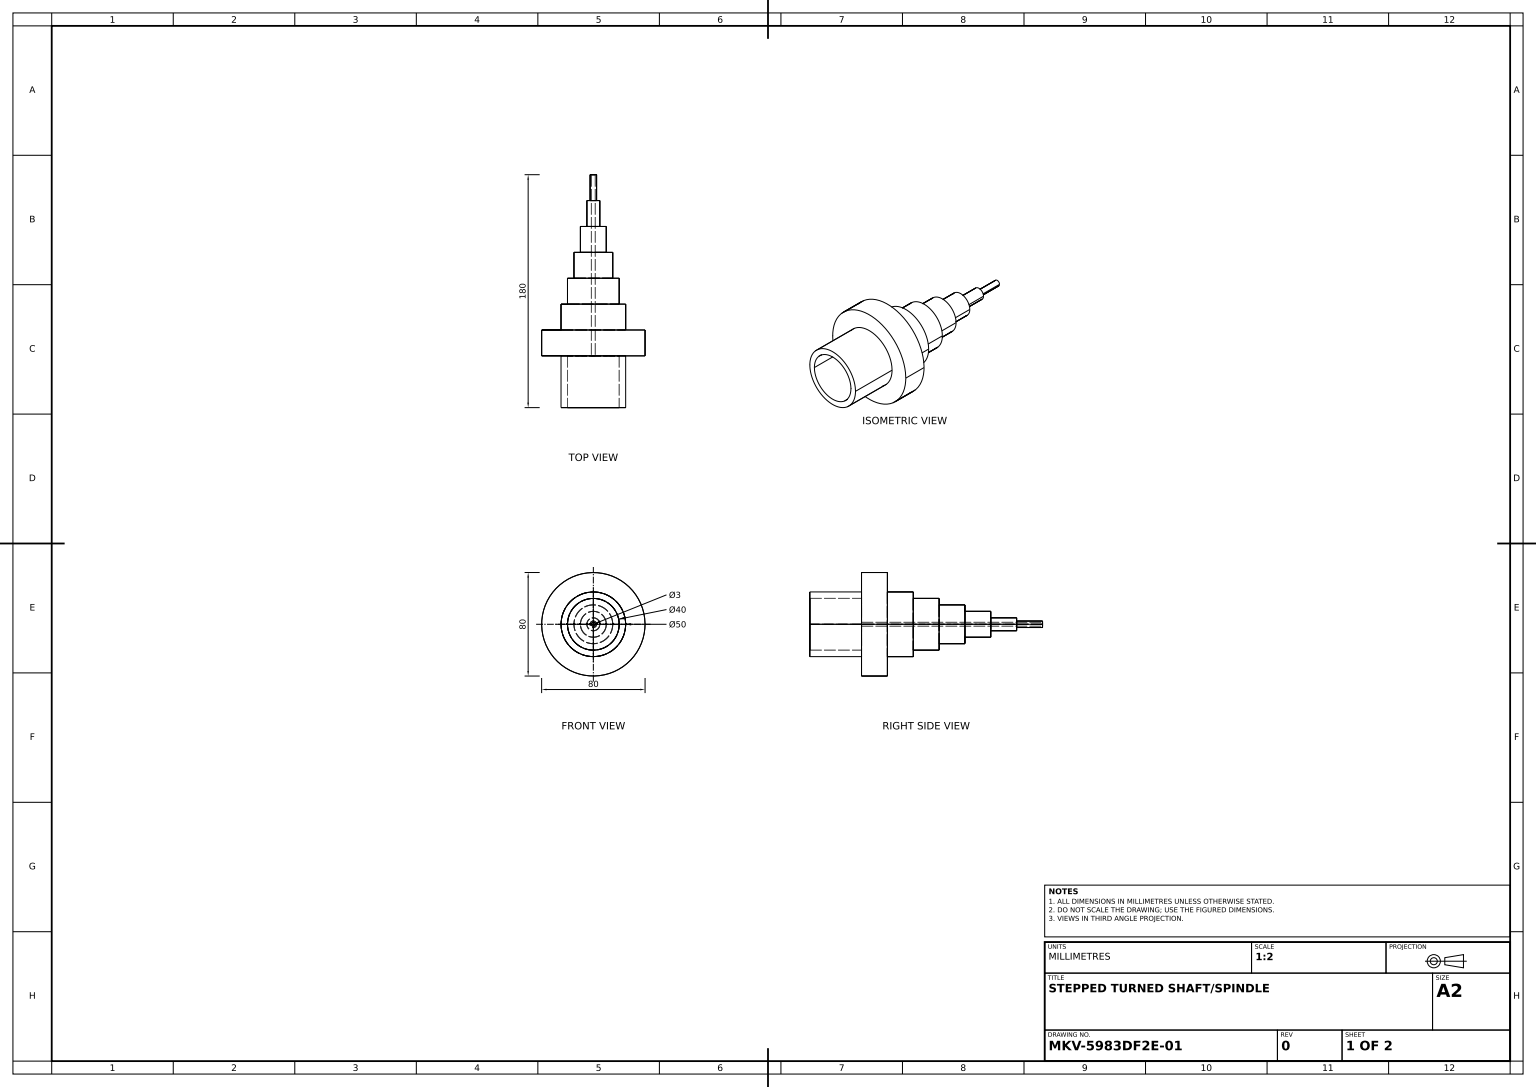
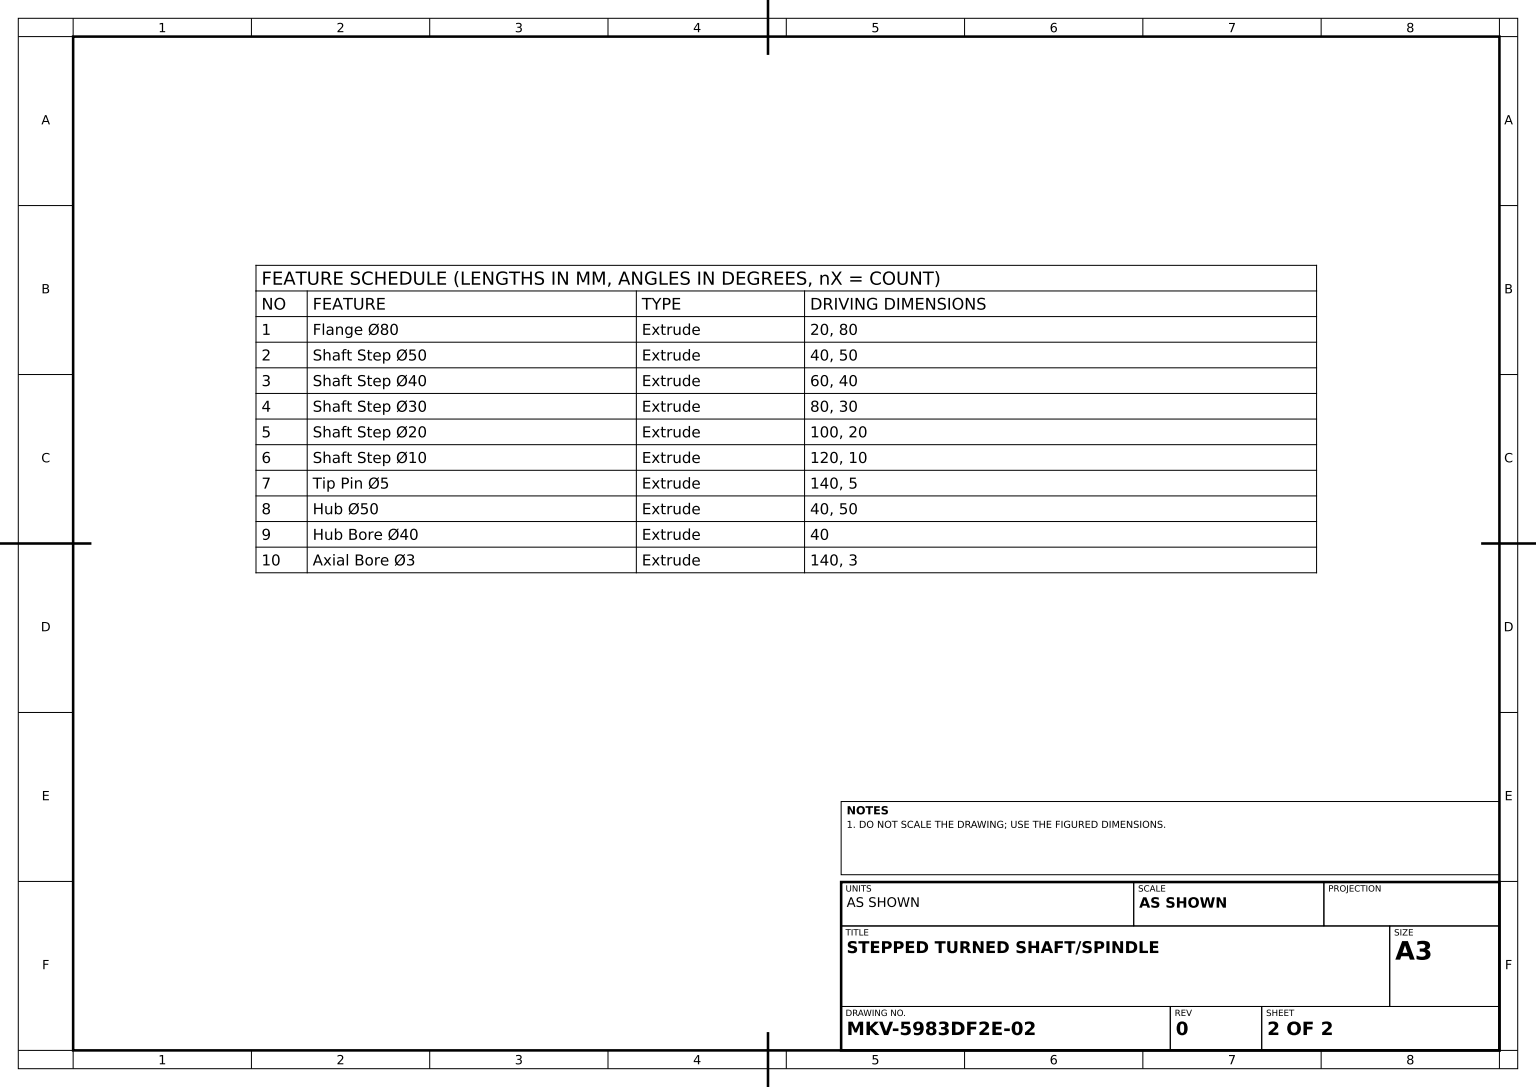
SolidWorks part; units mm, degrees
material "Plain Carbon Steel"
ref_plane "Front Plane" through (0, 0, 0) normal (0, 0, 1) x (1, 0, 0)
ref_plane "Top Plane" through (0, 0, 0) normal (0, 1, 0) x (1, 0, 0)
ref_plane "Right Plane" through (0, 0, 0) normal (1, 0, 0) x (0, 0, -1)
sketch "Flange Profile Ø80" plane through (0, 0, 0) normal (0, 0, 1) x (1, 0, 0)
  line L0 (0, 549.1728) -> (0, -534.2776) construction
  line L1 (-704.0777, 0) -> (998.442, 0) construction
  circle A0 centre (0, 0) radius 40
  dimension "D1" = 80
extrude "Flange Ø80" add sketch "Flange Profile Ø80" against normal blind 20
sketch "Step Ø50 Profile" plane through (0, 0, 0) normal (0, 0, 1) x (1, 0, 0)
  circle A0 centre (0, 0) radius 25
  dimension "D1" = 50
extrude "Shaft Step Ø50" add sketch "Step Ø50 Profile" against normal blind 40
sketch "Step Ø40 Profile" plane through (0, 0, 0) normal (0, 0, 1) x (1, 0, 0)
  circle A0 centre (0, 0) radius 20
  dimension "D1" = 40
extrude "Shaft Step Ø40" add sketch "Step Ø40 Profile" against normal blind 60
sketch "Step Ø30 Profile" plane through (0, 0, 0) normal (0, 0, 1) x (1, 0, 0)
  circle A0 centre (0, 0) radius 15
  dimension "D1" = 30
extrude "Shaft Step Ø30" add sketch "Step Ø30 Profile" against normal blind 80
sketch "Step Ø20 Profile" plane through (0, 0, 0) normal (0, 0, 1) x (1, 0, 0)
  circle A0 centre (0, 0) radius 10
  dimension "D1" = 20
extrude "Shaft Step Ø20" add sketch "Step Ø20 Profile" against normal blind 100
sketch "Step Ø10 Profile" plane through (0, 0, 0) normal (0, 0, 1) x (1, 0, 0)
  circle A0 centre (0, 0) radius 5
  dimension "D1" = 10
extrude "Shaft Step Ø10" add sketch "Step Ø10 Profile" against normal blind 120
sketch "Tip Pin Ø5 Profile" plane through (0, 0, 0) normal (0, 0, 1) x (1, 0, 0)
  circle A0 centre (0, 0) radius 2.5
  dimension "D1" = 5
extrude "Tip Pin Ø5" add sketch "Tip Pin Ø5 Profile" against normal blind 140
sketch "Hub Ø50 Profile" plane through (0, 0, 0) normal (0, 0, 1) x (1, 0, 0)
  circle A0 centre (0, 0) radius 25
  dimension "D1" = 50
extrude "Hub Ø50" add sketch "Hub Ø50 Profile" along normal blind 40
sketch "Hub Bore Ø40 Profile" plane through (0, 0, 40) normal (0, 0, 1) x (1, 0, 0)
  circle A0 centre (0, 0) radius 20
  dimension "D1" = 40
extrude "Hub Bore Ø40" cut sketch "Hub Bore Ø40 Profile" against normal blind 40
sketch "Axial Bore Ø3 Profile" plane through (0, 0, 0) normal (0, 0, 1) x (1, 0, 0)
  circle A0 centre (0, 0) radius 1.5
  dimension "D1" = 3
extrude "Axial Bore Ø3" cut sketch "Axial Bore Ø3 Profile" against normal blind 140
